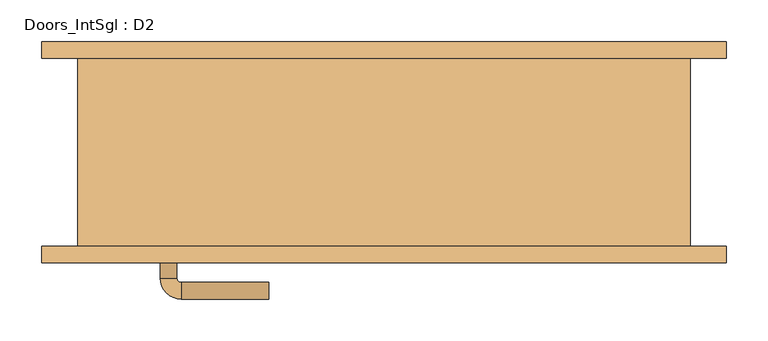
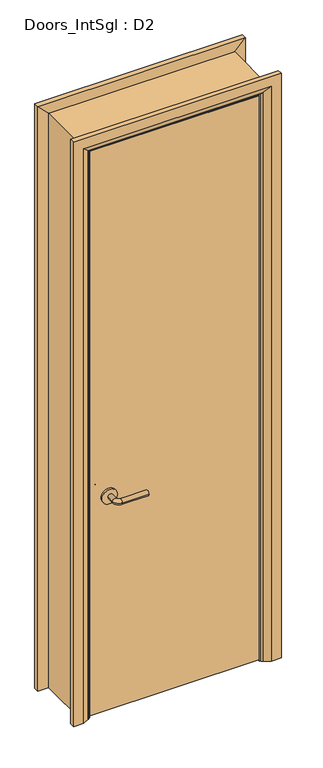
"""IFC4 building model written with IfcOpenShell, lengths in millimetres: door geometry, Doors_IntSgl : D2."""

from ifc_helpers import new_model, si_unit, point, frame, frame_2d, origin, place, context, project, spatial, polyline, circle_curve, ellipse_curve, trimmed, segment, composite_curve, outline, extrude, faceted_brep, source, transform, mapped, element, save
from ifc_brep_helpers import plane_surface, cylinder_surface, revolved_surface, advanced_brep


def doors_intsgl_d2_251e2544(model_context):
    return source(origin(), model_context, "Body", "SolidModel", [
        advanced_brep(
        [(-268.0, -66.5, 900.0), (-248.0, -66.5, 900.0), (-268.0, -36.5, 900.0), (-248.0, -36.5, 900.0), (-243.0, -31.5, 900.0), (-243.0, -11.5, 900.0), (-138.0, -11.5, 900.0), (-138.0, -31.5, 900.0)],
        [
            (0, 1, circle_curve(frame((-258.0, -66.5, 900.0), z_axis=(0.0, -1.0, 0.0), x_axis=(1.0, 0.0, 0.0)), 10.0)),
            (1, 0, circle_curve(frame((-258.0, -66.5, 900.0), z_axis=(0.0, -1.0, 0.0), x_axis=(1.0, 0.0, 0.0)), 10.0)),
            (0, 2),
            (2, 3, circle_curve(frame((-258.0, -36.5, 900.0), z_axis=(0.0, -1.0, 0.0), x_axis=(1.0, 0.0, 0.0)), 10.0)),
            (3, 1),
            (3, 2, circle_curve(frame((-258.0, -36.5, 900.0), z_axis=(0.0, -1.0, 0.0), x_axis=(1.0, 0.0, 0.0)), 10.0)),
            (4, 3, circle_curve(frame((-243.0, -36.5, 900.0), z_axis=(0.0, 0.0, 1.0), x_axis=(-1.0, 0.0, 0.0)), 5.0)),
            (2, 5, circle_curve(frame((-243.0, -36.5, 900.0), z_axis=(0.0, 0.0, -1.0), x_axis=(-1.0, 0.0, 0.0)), 25.0)),
            (5, 4, circle_curve(frame((-243.0, -21.5, 900.0), z_axis=(-1.0, 0.0, 0.0), x_axis=(0.0, -1.0, 0.0)), 10.0)),
            (4, 5, circle_curve(frame((-243.0, -21.5, 900.0), z_axis=(-1.0, 0.0, 0.0), x_axis=(0.0, -1.0, 0.0)), 10.0)),
            (6, 7, circle_curve(frame((-138.0, -21.5, 900.0), z_axis=(1.0, 0.0, 0.0), x_axis=(0.0, -1.0, 0.0)), 10.0)),
            (7, 6, circle_curve(frame((-138.0, -21.5, 900.0), z_axis=(1.0, 0.0, 0.0), x_axis=(0.0, -1.0, 0.0)), 10.0)),
            (5, 6),
            (7, 4),
        ],
        [
            plane_surface(frame((-258.0, -66.5, 900.0), z_axis=(0.0, -1.0, 0.0), x_axis=(0.0, 0.0, 1.0))),
            cylinder_surface(frame((-258.0, -66.5, 900.0), z_axis=(0.0, -1.0, 0.0), x_axis=(1.0, 0.0, 0.0)), 10.0),
            revolved_surface(trimmed(ellipse_curve(frame((-258.0, -36.5, 900.0), z_axis=(0.0, -1.0, 0.0), x_axis=(1.0, 0.0, 0.0)), 10.0, 10.0), [point((-268.0, -36.5, 900.0))], [point((-248.0, -36.5, 900.0))], True, "CARTESIAN"), (-243.0, -36.5, 900.0), (0.0, 0.0, -1.0)),
            revolved_surface(trimmed(ellipse_curve(frame((-258.0, -36.5, 900.0), z_axis=(0.0, -1.0, 0.0), x_axis=(1.0, 0.0, 0.0)), 10.0, 10.0), [point((-248.0, -36.5, 900.0))], [point((-268.0, -36.5, 900.0))], True, "CARTESIAN"), (-243.0, -36.5, 900.0), (0.0, 0.0, -1.0)),
            plane_surface(frame((-138.0, -21.5, 900.0), z_axis=(1.0, 0.0, 0.0), x_axis=(0.0, 0.0, 1.0))),
            cylinder_surface(frame((-243.0, -21.5, 900.0), z_axis=(-1.0, 0.0, 0.0), x_axis=(0.0, -1.0, 0.0)), 10.0),
        ],
        [
            (0, [[1, 2]]),
            (1, [[-1, 3, 4, 5]]),
            (1, [[-2, -5, 6, -3]]),
            (2, [[7, -4, 8, 9]]),
            (3, [[-8, -6, -7, 10]]),
            (4, [[11, 12]]),
            (5, [[-9, 13, -12, 14]]),
            (5, [[-10, -14, -11, -13]]),
        ],
    ),
        extrude(outline(composite_curve([segment(trimmed(circle_curve(frame_2d((900.0, -260.5)), 30.0), [point((900.0, -290.5))], [point((900.0, -230.5))], False, "CARTESIAN"), True, "CONTINUOUS"), segment(trimmed(circle_curve(frame_2d((900.0, -260.5)), 30.0), [point((900.0, -230.5))], [point((900.0, -290.5))], False, "CARTESIAN"), True, "CONTINUOUS")], self_intersect=False)), frame((0.0, -74.5, 0.0), z_axis=(0.0, 1.0, 0.0), x_axis=(0.0, 0.0, 1.0)), (0.0, 0.0, 1.0), 8.0),
        advanced_brep(
        [(-268.0, -120.5, 900.0), (-248.0, -120.5, 900.0), (-248.0, -150.5, 900.0), (-268.0, -150.5, 900.0), (-243.0, -155.5, 900.0), (-243.0, -175.5, 900.0), (-138.0, -175.5, 900.0), (-138.0, -155.5, 900.0)],
        [
            (0, 1, circle_curve(frame((-258.0, -120.5, 900.0), z_axis=(0.0, 1.0, 0.0), x_axis=(1.0, 0.0, 0.0)), 10.0)),
            (1, 0, circle_curve(frame((-258.0, -120.5, 900.0), z_axis=(0.0, 1.0, 0.0), x_axis=(1.0, 0.0, 0.0)), 10.0)),
            (1, 2),
            (2, 3, circle_curve(frame((-258.0, -150.5, 900.0), z_axis=(0.0, 1.0, 0.0), x_axis=(1.0, 0.0, 0.0)), 10.0)),
            (3, 0),
            (3, 2, circle_curve(frame((-258.0, -150.5, 900.0), z_axis=(0.0, 1.0, 0.0), x_axis=(1.0, 0.0, 0.0)), 10.0)),
            (4, 5, circle_curve(frame((-243.0, -165.5, 900.0), z_axis=(-1.0, 0.0, 0.0), x_axis=(0.0, 1.0, 0.0)), 10.0)),
            (5, 3, circle_curve(frame((-243.0, -150.5, 900.0), z_axis=(0.0, 0.0, -1.0), x_axis=(-1.0, 0.0, 0.0)), 25.0)),
            (2, 4, circle_curve(frame((-243.0, -150.5, 900.0), z_axis=(0.0, 0.0, 1.0), x_axis=(-1.0, 0.0, 0.0)), 5.0)),
            (5, 4, circle_curve(frame((-243.0, -165.5, 900.0), z_axis=(-1.0, 0.0, 0.0), x_axis=(0.0, 1.0, 0.0)), 10.0)),
            (6, 7, circle_curve(frame((-138.0, -165.5, 900.0), z_axis=(1.0, 0.0, 0.0), x_axis=(0.0, 1.0, 0.0)), 10.0)),
            (7, 6, circle_curve(frame((-138.0, -165.5, 900.0), z_axis=(1.0, 0.0, 0.0), x_axis=(0.0, 1.0, 0.0)), 10.0)),
            (4, 7),
            (6, 5),
        ],
        [
            plane_surface(frame((-258.0, -120.5, 900.0), z_axis=(0.0, 1.0, 0.0), x_axis=(0.0, 0.0, 1.0))),
            cylinder_surface(frame((-258.0, -120.5, 900.0), z_axis=(0.0, 1.0, 0.0), x_axis=(1.0, 0.0, 0.0)), 10.0),
            revolved_surface(trimmed(ellipse_curve(frame((-258.0, -150.5, 900.0), z_axis=(0.0, -1.0, 0.0), x_axis=(1.0, 0.0, 0.0)), 10.0, 10.0), [point((-268.0, -150.5, 900.0))], [point((-248.0, -150.5, 900.0))], True, "CARTESIAN"), (-243.0, -150.5, 900.0), (0.0, 0.0, -1.0)),
            revolved_surface(trimmed(ellipse_curve(frame((-258.0, -150.5, 900.0), z_axis=(0.0, -1.0, 0.0), x_axis=(1.0, 0.0, 0.0)), 10.0, 10.0), [point((-248.0, -150.5, 900.0))], [point((-268.0, -150.5, 900.0))], True, "CARTESIAN"), (-243.0, -150.5, 900.0), (0.0, 0.0, -1.0)),
            plane_surface(frame((-138.0, -165.5, 900.0), z_axis=(1.0, 0.0, 0.0), x_axis=(0.0, 0.0, 1.0))),
            cylinder_surface(frame((-243.0, -165.5, 900.0), z_axis=(-1.0, 0.0, 0.0), x_axis=(0.0, 1.0, 0.0)), 10.0),
        ],
        [
            (0, [[1, 2]]),
            (1, [[3, 4, 5, -2]]),
            (1, [[-5, 6, -3, -1]]),
            (2, [[7, 8, -4, 9]]),
            (3, [[10, -9, -6, -8]]),
            (4, [[11, 12]]),
            (5, [[13, -11, 14, -7]]),
            (5, [[-14, -12, -13, -10]]),
        ],
    ),
        extrude(outline(composite_curve([segment(trimmed(circle_curve(frame_2d((900.0, -260.5)), 30.0), [point((900.0, -290.5))], [point((900.0, -230.5))], False, "CARTESIAN"), True, "CONTINUOUS"), segment(trimmed(circle_curve(frame_2d((900.0, -260.5)), 30.0), [point((900.0, -230.5))], [point((900.0, -290.5))], False, "CARTESIAN"), True, "CONTINUOUS")], self_intersect=False)), frame((0.0, -120.5, 0.0), z_axis=(0.0, 1.0, 0.0), x_axis=(0.0, 0.0, 1.0)), (0.0, 0.0, 1.0), 8.0),
        extrude(outline(polyline([(333.0, -74.5), (333.0, -112.5), (-333.0, -112.5), (-333.0, -74.5), (333.0, -74.5)])), frame((0.0, 0.0, 8.0), z_axis=(0.0, 0.0, 1.0), x_axis=(1.0, 0.0, 0.0)), (0.0, 0.0, 1.0), 2350.0),
        faceted_brep([(-335.0, -112.5, 0.0), (-367.0, -112.5, 0.0), (-367.0, 112.5, 0.0), (-335.0, 112.5, 0.0), (-335.0, 112.5, 2360.0), (-335.0, -112.5, 2360.0), (-367.0, 112.5, 2392.0), (-367.0, -112.5, 2392.0), (335.0, -112.5, 0.0), (335.0, 112.5, 0.0), (367.0, 112.5, 0.0), (367.0, -112.5, 0.0), (335.0, -112.5, 2360.0), (367.0, -112.5, 2392.0), (367.0, 112.5, 2392.0), (335.0, 112.5, 2360.0)], [[[0, 1, 2, 3]], [[3, 4, 5, 0]], [[2, 6, 4, 3]], [[1, 7, 6, 2]], [[0, 5, 7, 1]], [[8, 9, 10, 11]], [[12, 8, 11, 13]], [[13, 11, 10, 14]], [[14, 10, 9, 15]], [[15, 9, 8, 12]], [[4, 15, 12, 5]], [[6, 14, 15, 4]], [[7, 13, 14, 6]], [[5, 12, 13, 7]]]),
        advanced_brep(
        [(-410.0, 132.5, 0.0), (-370.0, 132.5, 0.0), (-344.0, 118.5, 0.0), (-340.0, 112.5, 0.0), (-410.0, 112.5, 0.0), (-410.0, 112.5, 2435.0), (-410.0, 132.5, 2435.0), (-340.0, 112.5, 2365.0), (-344.0, 118.5, 2369.0), (-370.0, 132.5, 2395.0), (410.0, 132.5, 0.0), (410.0, 112.5, 0.0), (340.0, 112.5, 0.0), (344.0, 118.5, 0.0), (370.0, 132.5, 0.0), (410.0, 132.5, 2435.0), (370.0, 132.5, 2395.0), (344.0, 118.5, 2369.0), (340.0, 112.5, 2365.0), (410.0, 112.5, 2435.0)],
        [
            (0, 1),
            (1, 2),
            (2, 3, circle_curve(frame((-348.0, 111.5, 0.0), z_axis=(0.0, 0.0, -1.0), x_axis=(-1.0, 0.0, 0.0)), 8.0622577)),
            (3, 4),
            (4, 0),
            (4, 5),
            (5, 6),
            (6, 0),
            (3, 7),
            (7, 5),
            (2, 8),
            (8, 7, ellipse_curve(frame((-348.0, 111.5, 2373.0), z_axis=(-0.7071067811865475, 0.0, -0.7071067811865475), x_axis=(0.7071067811865474, 0.0, -0.7071067811865476)), 11.4017543, 8.0622577)),
            (1, 9),
            (9, 8),
            (6, 9),
            (10, 11),
            (11, 12),
            (12, 13, circle_curve(frame((348.0, 111.5, 0.0), z_axis=(0.0, 0.0, -1.0), x_axis=(1.0, 0.0, 0.0)), 8.0622577)),
            (13, 14),
            (14, 10),
            (15, 10),
            (14, 16),
            (16, 15),
            (13, 17),
            (17, 16),
            (12, 18),
            (18, 17, ellipse_curve(frame((348.0, 111.5, 2373.0), z_axis=(0.7071067811865475, 0.0, -0.7071067811865475), x_axis=(0.7071067811865474, 0.0, 0.7071067811865476)), 11.4017543, 8.0622577)),
            (11, 19),
            (19, 18),
            (15, 19),
            (5, 19),
            (15, 6),
            (7, 18),
            (8, 17),
            (9, 16),
        ],
        [
            plane_surface(frame((-340.0, 185.3010989, 0.0), z_axis=(0.0, 0.0, -1.0), x_axis=(1.0, 0.0, 0.0))),
            plane_surface(frame((-410.0, 132.5, 0.0), z_axis=(-1.0, 0.0, 0.0), x_axis=(0.0, 0.0, 1.0))),
            plane_surface(frame((-410.0, 112.5, 0.0), z_axis=(0.0, -1.0, 0.0), x_axis=(0.0, 0.0, 1.0))),
            cylinder_surface(frame((-348.0, 111.5, 0.0), z_axis=(0.0, 0.0, -1.0), x_axis=(-1.0, 0.0, 0.0)), 8.0622577),
            plane_surface(frame((-344.0, 118.5, 0.0), z_axis=(0.4740998230350183, 0.8804710999221749, 0.0), x_axis=(0.0, 0.0, 1.0))),
            plane_surface(frame((-370.0, 132.5, 0.0), z_axis=(0.0, 1.0, 0.0), x_axis=(0.0, 0.0, 1.0))),
            plane_surface(frame((340.0, 185.3010989, 0.0), z_axis=(0.0, 0.0, -1.0), x_axis=(-1.0, 0.0, 0.0))),
            plane_surface(frame((370.0, 132.5, 2395.0), z_axis=(0.0, 1.0, 0.0), x_axis=(0.0, 0.0, -1.0))),
            plane_surface(frame((344.0, 118.5, 2369.0), z_axis=(-0.4740998230350183, 0.8804710999221749, 0.0), x_axis=(0.0, 0.0, -1.0))),
            cylinder_surface(frame((348.0, 111.5, 2365.0), z_axis=(0.0, 0.0, 1.0), x_axis=(1.0, 0.0, 0.0)), 8.0622577),
            plane_surface(frame((410.0, 112.5, 2435.0), z_axis=(0.0, -1.0, 0.0), x_axis=(0.0, 0.0, -1.0))),
            plane_surface(frame((410.0, 132.5, 2435.0), z_axis=(1.0, 0.0, 0.0), x_axis=(0.0, 0.0, -1.0))),
            plane_surface(frame((-410.0, 132.5, 2435.0), z_axis=(0.0, 0.0, 1.0), x_axis=(1.0, 0.0, 0.0))),
            plane_surface(frame((-410.0, 112.5, 2435.0), z_axis=(0.0, -1.0, 0.0), x_axis=(1.0, 0.0, 0.0))),
            cylinder_surface(frame((-340.0, 111.5, 2373.0), z_axis=(-1.0, 0.0, 0.0), x_axis=(0.0, 0.0, 1.0)), 8.0622577),
            plane_surface(frame((-344.0, 118.5, 2369.0), z_axis=(0.0, 0.8804710999221749, -0.4740998230350183), x_axis=(1.0, 0.0, 0.0))),
            plane_surface(frame((-370.0, 132.5, 2395.0), z_axis=(0.0, 1.0, 0.0), x_axis=(1.0, 0.0, 0.0))),
        ],
        [
            (0, [[1, 2, 3, 4, 5]]),
            (1, [[6, 7, 8, -5]]),
            (2, [[9, 10, -6, -4]]),
            (3, [[11, 12, -9, -3]]),
            (4, [[13, 14, -11, -2]]),
            (5, [[-8, 15, -13, -1]]),
            (6, [[16, 17, 18, 19, 20]]),
            (7, [[21, -20, 22, 23]]),
            (8, [[-22, -19, 24, 25]]),
            (9, [[-24, -18, 26, 27]]),
            (10, [[-26, -17, 28, 29]]),
            (11, [[-28, -16, -21, 30]]),
            (12, [[31, -30, 32, -7]]),
            (13, [[33, -29, -31, -10]]),
            (14, [[34, -27, -33, -12]]),
            (15, [[35, -25, -34, -14]]),
            (16, [[-32, -23, -35, -15]]),
        ],
    ),
        extrude(outline(polyline([(0.0, -316.0), (2341.0, -316.0), (2341.0, 316.0), (0.0, 316.0), (0.0, 335.0), (2360.0, 335.0), (2360.0, -335.0), (0.0, -335.0), (0.0, -316.0)])), frame((0.0, -72.5, 0.0), z_axis=(0.0, 1.0, 0.0), x_axis=(0.0, 0.0, 1.0)), (0.0, 0.0, 1.0), 32.0),
        advanced_brep(
        [(410.0, -132.5, 0.0), (370.0, -132.5, 0.0), (344.0, -118.5, 0.0), (340.0, -112.5, 0.0), (410.0, -112.5, 0.0), (410.0, -112.5, 2435.0), (410.0, -132.5, 2435.0), (340.0, -112.5, 2365.0), (-340.0, -112.5, 2365.0), (-340.0, -112.5, 0.0), (-410.0, -112.5, 0.0), (-410.0, -112.5, 2435.0), (344.0, -118.5, 2369.0), (370.0, -132.5, 2395.0), (-410.0, -132.5, 2435.0), (-410.0, -132.5, 0.0), (-370.0, -132.5, 0.0), (-370.0, -132.5, 2395.0), (-344.0, -118.5, 0.0), (-344.0, -118.5, 2369.0)],
        [
            (0, 1),
            (1, 2),
            (2, 3, circle_curve(frame((348.0, -111.5, 0.0), z_axis=(0.0, 0.0, -1.0), x_axis=(1.0, 0.0, 0.0)), 8.0622577)),
            (3, 4),
            (4, 0),
            (4, 5),
            (5, 6),
            (6, 0),
            (3, 7),
            (7, 8),
            (8, 9),
            (9, 10),
            (10, 11),
            (11, 5),
            (2, 12),
            (12, 7, ellipse_curve(frame((348.0, -111.5, 2373.0), z_axis=(0.7071067811865475, 0.0, -0.7071067811865475), x_axis=(-0.7071067811865474, 0.0, -0.7071067811865476)), 11.4017543, 8.0622577)),
            (1, 13),
            (13, 12),
            (6, 14),
            (14, 15),
            (15, 16),
            (16, 17),
            (17, 13),
            (10, 15),
            (14, 11),
            (9, 18, circle_curve(frame((-348.0, -111.5, 0.0), z_axis=(0.0, 0.0, -1.0), x_axis=(-1.0, 0.0, 0.0)), 8.0622577)),
            (18, 16),
            (19, 18),
            (8, 19, ellipse_curve(frame((-348.0, -111.5, 2373.0), z_axis=(-0.7071067811865475, 0.0, -0.7071067811865475), x_axis=(-0.7071067811865474, 0.0, 0.7071067811865476)), 11.4017543, 8.0622577)),
            (19, 17),
            (12, 19),
        ],
        [
            plane_surface(frame((340.0, -112.5, 0.0), z_axis=(0.0, 0.0, -1.0), x_axis=(0.0, 1.0, 0.0))),
            plane_surface(frame((410.0, -132.5, 0.0), z_axis=(1.0, 0.0, 0.0), x_axis=(0.0, 0.0, 1.0))),
            plane_surface(frame((410.0, -112.5, 0.0), z_axis=(0.0, 1.0, 0.0), x_axis=(0.0, 0.0, 1.0))),
            cylinder_surface(frame((348.0, -111.5, 0.0), z_axis=(0.0, 0.0, -1.0), x_axis=(1.0, 0.0, 0.0)), 8.0622577),
            plane_surface(frame((344.0, -118.5, 0.0), z_axis=(-0.4740998230350126, -0.880471099922178, 0.0), x_axis=(0.0, 0.0, 1.0))),
            plane_surface(frame((370.0, -132.5, 0.0), z_axis=(0.0, -1.0, 0.0), x_axis=(0.0, 0.0, 1.0))),
            plane_surface(frame((-410.0, -132.5, 2435.0), z_axis=(-1.0, 0.0, 0.0), x_axis=(0.0, 0.0, -1.0))),
            plane_surface(frame((-340.0, -112.5, 0.0), z_axis=(0.0, 0.0, -1.0), x_axis=(0.0, 1.0, 0.0))),
            cylinder_surface(frame((-348.0, -111.5, 2365.0), z_axis=(0.0, 0.0, 1.0), x_axis=(-1.0, 0.0, 0.0)), 8.0622577),
            plane_surface(frame((-344.0, -118.5, 2369.0), z_axis=(0.47409982303501824, -0.8804710999221749, 0.0), x_axis=(0.0, 0.0, -1.0))),
            plane_surface(frame((410.0, -132.5, 2435.0), z_axis=(0.0, 0.0, 1.0), x_axis=(-1.0, 0.0, 0.0))),
            cylinder_surface(frame((340.0, -111.5, 2373.0), z_axis=(1.0, 0.0, 0.0), x_axis=(0.0, 0.0, 1.0)), 8.0622577),
            plane_surface(frame((344.0, -118.5, 2369.0), z_axis=(0.0, -0.8804710999221764, -0.4740998230350154), x_axis=(-1.0, 0.0, 0.0))),
        ],
        [
            (0, [[1, 2, 3, 4, 5]]),
            (1, [[6, 7, 8, -5]]),
            (2, [[9, 10, 11, 12, 13, 14, -6, -4]]),
            (3, [[15, 16, -9, -3]]),
            (4, [[17, 18, -15, -2]]),
            (5, [[-8, 19, 20, 21, 22, 23, -17, -1]]),
            (6, [[-13, 24, -20, 25]]),
            (7, [[-24, -12, 26, 27, -21]]),
            (8, [[28, -26, -11, 29]]),
            (9, [[-22, -27, -28, 30]]),
            (10, [[-14, -25, -19, -7]]),
            (11, [[31, -29, -10, -16]]),
            (12, [[-23, -30, -31, -18]]),
        ],
    ),
    ])


if __name__ == "__main__":
    model = new_model("IFC4")
    model_context = context("Model", 3, world=origin())
    ifc_project = project(units=[si_unit("LENGTHUNIT", "METRE", prefix="MILLI")], contexts=[model_context])
    site = spatial("IfcSite", under=ifc_project)
    building = spatial("IfcBuilding", under=site)
    placement = place(None, origin())
    doors_intsgl_d2_shape = doors_intsgl_d2_251e2544(model_context)
    element("IfcDoor", 1, ObjectType="Doors_IntSgl : D2", at=placement, inside=building, context=model_context, shape_type="MappedRepresentation", body=[
        mapped(doors_intsgl_d2_shape, transform((0.0, 0.0, 0.0), x_axis=(1.0, 0.0, 0.0), y_axis=(0.0, 1.0, 0.0), z_axis=(0.0, 0.0, 1.0))),
    ])
    save(model, "model.ifc")

# Revit data of these elements
# Type "Doors_IntSgl : D2"
#   Type Mark = "52"
#   Type Comments = "Internal Single"
#   Operation = "SingleSwingRight"
#   Manufacturer = "Revit"
#   Keynote = "L20"
#   Description = "Internal Single Door"
#   Analytic Construction = "Metal"
#   UnderCut = 8 mm
#   Tolerance = 2 mm
#   Thickness = 38 mm
#   Thermal Resistance (R) = 0.270117 (m²·K)/W
#   Structural Tolerance = 8 mm
#   StopDepth = 32 mm
#   Stop Thickness = 19 mm
#   Rough Width = 750 mm
#   Rough Height = 2400 mm
#   Height to Top Lock Rail = 1000 mm
#   Heat Transfer Coefficient (U) = 3.7021 W/(m²·K)
#   Handle Z Distance = 900 mm
#   Handle X Distance = 75 mm
#   Frame Thickness = 32 mm
#   Door Panel Width = 666 mm
#   Door Panel Thickness = 38 mm
#   Door Panel Offset = 0 mm
#   Height = 2400 mm
#   Width = 750 mm
#   Door Panel Height = 2350 mm
#   Architrave Setback = 5 mm
#   Vis - Ironmongery = yes
#   Define Thermal Properties by = 1
#   Material Ironmongery = Door - Handle
#   Material Frame = Door - Frame/Mullion (1)
#   Material Door = Door - Panel
#   Material Architrave = Door - Architrave
#   Visual Light Transmittance = 0
#   Solar Heat Gain Coefficient = 0
#   Function = (empty or 0)
#   Wall Closure = (empty or 0)
# Element 1 (IfcDoor, "Doors_IntSgl : D2")
#   Materials on its faces: "Door - Architrave", "Door - Handle", "Door - Frame/Mullion (1)", "Door - Panel"
# Materials
#   "Door - Handle": colour RGB 0 0 0, transparency 0, Keynote = "P21", Cost = 0
#   "Door - Frame/Mullion (1)": class "Wood", colour RGB 212 179 113, transparency 0, Keynote = "L20", Cost = 0
#   "Door - Panel": class "Wood", colour RGB 210 159 95, transparency 0, Keynote = "L20", Cost = 0
#   "Door - Architrave": class "Wood", colour RGB 154 90 5, transparency 0, Keynote = "P20", Cost = 0
